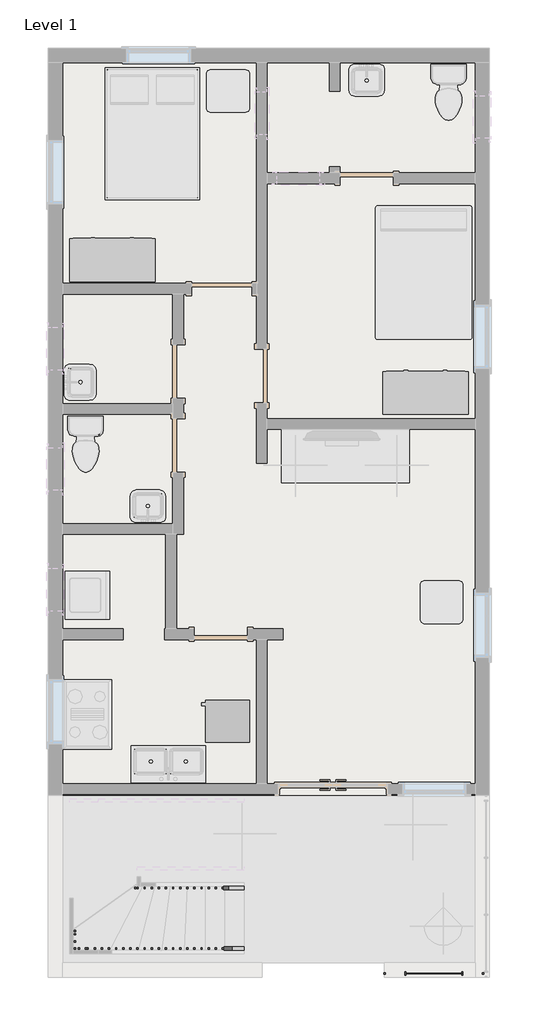
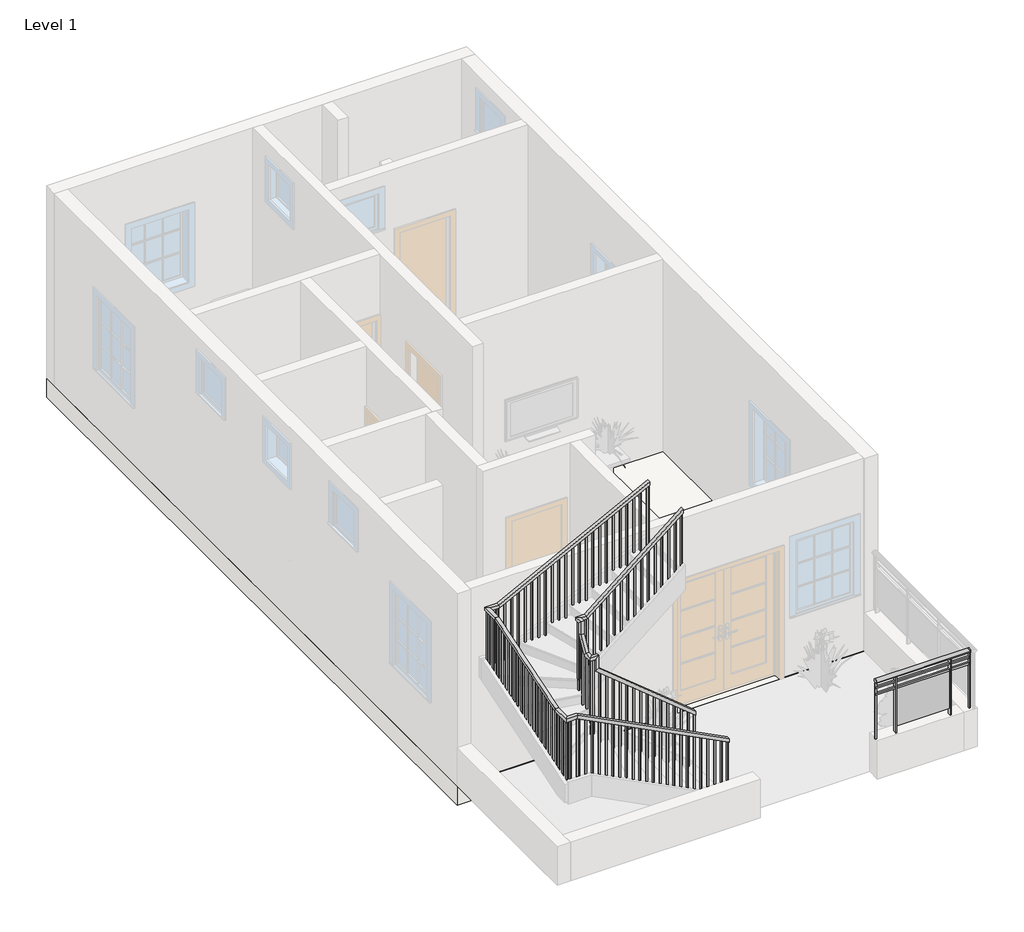
# One storey, part 2 of 3: 3 railings, 1 slab.
"""IFC4 building model written with IfcOpenShell, lengths in millimetres."""

from ifc_helpers import new_model, si_unit, point, frame, origin, place, context, project, spatial, polyline, ellipse_curve, trimmed, outline, extrude, faceted_brep, element, save
from ifc_brep_helpers import plane_surface, extruded_surface, advanced_brep

model = new_model("IFC4")

# Units and contexts
model_context = context("Model", 3, world=origin())
ifc_project = project(units=[si_unit("LENGTHUNIT", "METRE", prefix="MILLI")], contexts=[model_context])

# Site, building, storey
site = spatial("IfcSite", under=ifc_project)
building = spatial("IfcBuilding", under=site)
storey = spatial("IfcBuildingStorey", under=building, Name="Level 1", Elevation=0.0)

# Railings
placement = place(None, origin())
element("IfcRailing", 1, ObjectType="Glass Panel - Bottom Fill", at=placement, inside=storey, context=model_context, shape_type="SolidModel", body=[
    advanced_brep(
    [(-9850.6560632, 3087.8418963, 1524.0), (-9850.6560632, 3164.0418963, 1524.0), (-11259.7757671, 3087.8418963, 1524.0), (-11259.7757671, 3164.0418963, 1524.0)],
    [
        (0, 1, ellipse_curve(frame((-9850.6560632, 3125.9418963, 1524.0), z_axis=(1.0, 0.0, 0.0), x_axis=(0.0, 1.0, 0.0)), 38.1, 28.575)),
        (1, 0, ellipse_curve(frame((-9850.6560632, 3125.9418963, 1524.0), z_axis=(1.0, 0.0, 0.0), x_axis=(0.0, 1.0, 0.0)), 38.1, 28.575)),
        (2, 3, ellipse_curve(frame((-11259.7757671, 3125.9418963, 1524.0), z_axis=(-1.0, 0.0, 0.0), x_axis=(0.0, 1.0, 0.0)), 38.1, 28.575)),
        (3, 2, ellipse_curve(frame((-11259.7757671, 3125.9418963, 1524.0), z_axis=(-1.0, 0.0, 0.0), x_axis=(0.0, 1.0, 0.0)), 38.1, 28.575)),
        (0, 2),
        (3, 1),
    ],
    [
        plane_surface(frame((-9850.6560632, 3125.9418963, 1524.0), z_axis=(1.0, 0.0, 0.0), x_axis=(0.0, -1.0, 0.0))),
        plane_surface(frame((-11259.7757671, 3125.9418963, 1524.0), z_axis=(-1.0, 0.0, 0.0), x_axis=(0.0, -1.0, 0.0))),
        extruded_surface(trimmed(ellipse_curve(frame((-11259.7757671, 3125.9418963, 1524.0), z_axis=(1.0, 0.0, 0.0), x_axis=(0.0, 1.0, 0.0)), 38.1, 28.575), [point((-11259.7757671, 3087.8418963, 1524.0))], [point((-11259.7757671, 3164.0418963, 1524.0))], True, "CARTESIAN"), (1409.1197038999999, 0.0, 0.0), 1409.1197038999999),
        extruded_surface(trimmed(ellipse_curve(frame((-11259.7757671, 3125.9418963, 1524.0), z_axis=(1.0, 0.0, 0.0), x_axis=(0.0, 1.0, 0.0)), 38.1, 28.575), [point((-11259.7757671, 3164.0418963, 1524.0))], [point((-11259.7757671, 3087.8418963, 1524.0))], True, "CARTESIAN"), (1409.1197038999999, 0.0, 0.0), 1409.1197038999999),
    ],
    [
        (0, [[1, 2]]),
        (1, [[3, 4]]),
        (2, [[-1, 5, -4, 6]]),
        (3, [[-2, -6, -3, -5]]),
    ],
),
    extrude(outline(polyline([(-9850.6560632, 3138.6418963), (-9850.6560632, 3113.2418963), (-11259.7757671, 3113.2418963), (-11259.7757671, 3138.6418963), (-9850.6560632, 3138.6418963)])), frame((0.0, 0.0, 1409.7), z_axis=(0.0, 0.0, 1.0), x_axis=(1.0, 0.0, 0.0)), (0.0, 0.0, 1.0), 25.4),
    extrude(outline(polyline([(-9850.6560632, 3138.6418963), (-9850.6560632, 3113.2418963), (-11259.7757671, 3113.2418963), (-11259.7757671, 3138.6418963), (-9850.6560632, 3138.6418963)])), frame((0.0, 0.0, 1308.1), z_axis=(0.0, 0.0, 1.0), x_axis=(1.0, 0.0, 0.0)), (0.0, 0.0, 1.0), 25.4),
    extrude(outline(polyline([(-10955.2659151, 3151.3418963), (-10955.2659151, 3100.5418963), (-10967.9659151, 3100.5418963), (-10967.9659151, 3151.3418963), (-10955.2659151, 3151.3418963)])), frame((0.0, 0.0, 609.6), z_axis=(0.0, 0.0, 1.0), x_axis=(1.0, 0.0, 0.0)), (0.0, 0.0, 1.0), 885.6788223),
    extrude(outline(polyline([(-10148.8159151, 3119.4067393), (-10961.6159151, 3119.4067393), (-10961.6159151, 3125.7567393), (-10148.8159151, 3125.7567393), (-10148.8159151, 3119.4067393)])), frame((0.0, 0.0, 711.2), z_axis=(0.0, 0.0, 1.0), x_axis=(1.0, 0.0, 0.0)), (0.0, 0.0, 1.0), 596.9),
    extrude(outline(polyline([(-10142.4659151, 3151.3418963), (-10142.4659151, 3100.5418963), (-10155.1659151, 3100.5418963), (-10155.1659151, 3151.3418963), (-10142.4659151, 3151.3418963)])), frame((0.0, 0.0, 609.6), z_axis=(0.0, 0.0, 1.0), x_axis=(1.0, 0.0, 0.0)), (0.0, 0.0, 1.0), 885.6788223),
    extrude(outline(polyline([(-11247.0757671, 3135.4668963), (-11247.0757671, 3116.4168963), (-11266.1257671, 3116.4168963), (-11266.1257671, 3135.4668963), (-11247.0757671, 3135.4668963)])), frame((0.0, 0.0, 609.6), z_axis=(0.0, 0.0, 1.0), x_axis=(1.0, 0.0, 0.0)), (0.0, 0.0, 1.0), 885.6788223),
    extrude(outline(polyline([(-9844.3060632, 3135.4668963), (-9844.3060632, 3116.4168963), (-9863.3560632, 3116.4168963), (-9863.3560632, 3135.4668963), (-9844.3060632, 3135.4668963)])), frame((0.0, 0.0, 609.6), z_axis=(0.0, 0.0, 1.0), x_axis=(1.0, 0.0, 0.0)), (0.0, 0.0, 1.0), 885.6788223),
])
element("IfcRailing", 2, ObjectType="Handrail - Rectangular", at=placement, inside=storey, context=model_context, shape_type="SolidModel", body=[
    faceted_brep([(-13262.6440752, 4319.7418963, 1025.2529681), (-13262.6440752, 4319.7418963, 959.7067088), (-13262.6440752, 4370.5418963, 959.7067088), (-13262.6440752, 4370.5418963, 1025.2529681), (-14714.1757671, 4319.7418963, 2208.7848338), (-14764.9757671, 4319.7418963, 2184.659247), (-14764.9757671, 4370.5418963, 2184.659247), (-14714.1757671, 4370.5418963, 2208.7848338), (-14714.1757671, 4319.7418963, 2414.6281882), (-14764.9757671, 4319.7418963, 2363.8281882), (-14764.9757671, 4370.5418963, 2363.8281882), (-14714.1757671, 4370.5418963, 2414.6281882), (-14841.1757671, 4319.7418963, 2414.6281882), (-14841.1757671, 4319.7418963, 2363.8281882), (-14790.3757671, 4370.5418963, 2363.8281882), (-14790.3757671, 4370.5418963, 2414.6281882), (-14841.1757671, 4446.7418963, 2414.6281882), (-14841.1757671, 4475.8632301, 2363.8281882), (-14790.3757671, 4475.8632301, 2363.8281882), (-14790.3757671, 4446.7418963, 2414.6281882), (-14841.1757671, 4573.7418963, 2631.5051451), (-14841.1757671, 4624.5418963, 2617.7256424), (-14790.3757671, 4624.5418963, 2617.7256424), (-14790.3757671, 4573.7418963, 2631.5051451), (-14841.1757671, 4573.7418963, 2837.3484995), (-14841.1757671, 4624.5418963, 2786.5484995), (-14790.3757671, 4624.5418963, 2786.5484995), (-14790.3757671, 4573.7418963, 2837.3484995), (-14841.1757671, 4700.7418963, 2837.3484995), (-14841.1757671, 4700.7418963, 2786.5484995), (-14790.3757671, 4649.9418963, 2786.5484995), (-14790.3757671, 4649.9418963, 2837.3484995), (-14714.1757671, 4700.7418963, 2837.3484995), (-14696.090354, 4700.7418963, 2786.5484995), (-14696.090354, 4649.9418963, 2786.5484995), (-14714.1757671, 4649.9418963, 2837.3484995), (-13262.6440752, 4700.7418963, 4020.8803652), (-13262.6440752, 4649.9418963, 4020.8803652), (-13262.6440752, 4649.9418963, 3955.3341059), (-13262.6440752, 4700.7418963, 3955.3341059)], [[[0, 1, 2, 3]], [[1, 0, 4, 5]], [[2, 1, 5, 6]], [[3, 2, 6, 7]], [[0, 3, 7, 4]], [[5, 4, 8, 9]], [[6, 5, 9, 10]], [[7, 6, 10, 11]], [[4, 7, 11, 8]], [[9, 8, 12, 13]], [[10, 9, 13, 14]], [[11, 10, 14, 15]], [[8, 11, 15, 12]], [[13, 12, 16, 17]], [[14, 13, 17, 18]], [[15, 14, 18, 19]], [[12, 15, 19, 16]], [[17, 16, 20, 21]], [[18, 17, 21, 22]], [[19, 18, 22, 23]], [[16, 19, 23, 20]], [[21, 20, 24, 25]], [[22, 21, 25, 26]], [[23, 22, 26, 27]], [[20, 23, 27, 24]], [[25, 24, 28, 29]], [[26, 25, 29, 30]], [[27, 26, 30, 31]], [[24, 27, 31, 28]], [[29, 28, 32, 33]], [[30, 29, 33, 34]], [[31, 30, 34, 35]], [[28, 31, 35, 32]], [[36, 37, 38, 39]], [[33, 32, 36, 39]], [[34, 33, 39, 38]], [[35, 34, 38, 37]], [[32, 35, 37, 36]]]),
    extrude(outline(polyline([(3881.7558784, -13352.8834107), (3866.2231262, -13371.9334107), (2878.6666667, -13371.9334107), (2878.6666667, -13352.8834107), (3881.7558784, -13352.8834107)])), frame((0.0, 4665.8168963, 0.0), z_axis=(0.0, 1.0, 0.0), x_axis=(0.0, 0.0, 1.0)), (0.0, 0.0, 1.0), 19.05),
    extrude(outline(polyline([(3798.9145334, -13454.4834107), (3783.3817813, -13473.5334107), (2878.6666667, -13473.5334107), (2878.6666667, -13454.4834107), (3798.9145334, -13454.4834107)])), frame((0.0, 4665.8168963, 0.0), z_axis=(0.0, 1.0, 0.0), x_axis=(0.0, 0.0, 1.0)), (0.0, 0.0, 1.0), 19.05),
    extrude(outline(polyline([(3716.0731885, -13556.0834107), (3700.5404364, -13575.1334107), (2709.3333333, -13575.1334107), (2709.3333333, -13556.0834107), (3716.0731885, -13556.0834107)])), frame((0.0, 4665.8168963, 0.0), z_axis=(0.0, 1.0, 0.0), x_axis=(0.0, 0.0, 1.0)), (0.0, 0.0, 1.0), 19.05),
    extrude(outline(polyline([(3633.2318436, -13657.6834107), (3617.6990914, -13676.7334107), (2709.3333333, -13676.7334107), (2709.3333333, -13657.6834107), (3633.2318436, -13657.6834107)])), frame((0.0, 4665.8168963, 0.0), z_axis=(0.0, 1.0, 0.0), x_axis=(0.0, 0.0, 1.0)), (0.0, 0.0, 1.0), 19.05),
    extrude(outline(polyline([(3550.3904987, -13759.2834107), (3534.8577465, -13778.3334107), (2709.3333333, -13778.3334107), (2709.3333333, -13759.2834107), (3550.3904987, -13759.2834107)])), frame((0.0, 4665.8168963, 0.0), z_axis=(0.0, 1.0, 0.0), x_axis=(0.0, 0.0, 1.0)), (0.0, 0.0, 1.0), 19.05),
    extrude(outline(polyline([(3467.5491538, -13860.8834107), (3452.0164016, -13879.9334107), (2540.0, -13879.9334107), (2540.0, -13860.8834107), (3467.5491538, -13860.8834107)])), frame((0.0, 4665.8168963, 0.0), z_axis=(0.0, 1.0, 0.0), x_axis=(0.0, 0.0, 1.0)), (0.0, 0.0, 1.0), 19.05),
    extrude(outline(polyline([(3384.7078088, -13962.4834107), (3369.1750567, -13981.5334107), (2540.0, -13981.5334107), (2540.0, -13962.4834107), (3384.7078088, -13962.4834107)])), frame((0.0, 4665.8168963, 0.0), z_axis=(0.0, 1.0, 0.0), x_axis=(0.0, 0.0, 1.0)), (0.0, 0.0, 1.0), 19.05),
    extrude(outline(polyline([(3301.8664639, -14064.0834107), (3286.3337117, -14083.1334107), (2540.0, -14083.1334107), (2540.0, -14064.0834107), (3301.8664639, -14064.0834107)])), frame((0.0, 4665.8168963, 0.0), z_axis=(0.0, 1.0, 0.0), x_axis=(0.0, 0.0, 1.0)), (0.0, 0.0, 1.0), 19.05),
    extrude(outline(polyline([(3219.025119, -14165.6834107), (3203.4923668, -14184.7334107), (2370.6666667, -14184.7334107), (2370.6666667, -14165.6834107), (3219.025119, -14165.6834107)])), frame((0.0, 4665.8168963, 0.0), z_axis=(0.0, 1.0, 0.0), x_axis=(0.0, 0.0, 1.0)), (0.0, 0.0, 1.0), 19.05),
    extrude(outline(polyline([(3136.1837741, -14267.2834107), (3120.6510219, -14286.3334107), (2370.6666667, -14286.3334107), (2370.6666667, -14267.2834107), (3136.1837741, -14267.2834107)])), frame((0.0, 4665.8168963, 0.0), z_axis=(0.0, 1.0, 0.0), x_axis=(0.0, 0.0, 1.0)), (0.0, 0.0, 1.0), 19.05),
    extrude(outline(polyline([(3053.3424291, -14368.8834107), (3037.809677, -14387.9334107), (2201.3333333, -14387.9334107), (2201.3333333, -14368.8834107), (3053.3424291, -14368.8834107)])), frame((0.0, 4665.8168963, 0.0), z_axis=(0.0, 1.0, 0.0), x_axis=(0.0, 0.0, 1.0)), (0.0, 0.0, 1.0), 19.05),
    extrude(outline(polyline([(2970.5010842, -14470.4834107), (2954.9683321, -14489.5334107), (2201.3333333, -14489.5334107), (2201.3333333, -14470.4834107), (2970.5010842, -14470.4834107)])), frame((0.0, 4665.8168963, 0.0), z_axis=(0.0, 1.0, 0.0), x_axis=(0.0, 0.0, 1.0)), (0.0, 0.0, 1.0), 19.05),
    extrude(outline(polyline([(2887.6597393, -14572.0834107), (2872.1269871, -14591.1334107), (2032.0, -14591.1334107), (2032.0, -14572.0834107), (2887.6597393, -14572.0834107)])), frame((0.0, 4665.8168963, 0.0), z_axis=(0.0, 1.0, 0.0), x_axis=(0.0, 0.0, 1.0)), (0.0, 0.0, 1.0), 19.05),
    extrude(outline(polyline([(2804.8183944, -14673.6834107), (2789.2856422, -14692.7334107), (2032.0, -14692.7334107), (2032.0, -14673.6834107), (2804.8183944, -14673.6834107)])), frame((0.0, 4665.8168963, 0.0), z_axis=(0.0, 1.0, 0.0), x_axis=(0.0, 0.0, 1.0)), (0.0, 0.0, 1.0), 19.05),
    extrude(outline(polyline([(4553.6028, 2496.5834745), (4572.6528, 2529.115018), (4572.6528, 1524.0), (4553.6028, 1524.0), (4553.6028, 2496.5834745)])), frame((-14825.3007671, 0.0, 0.0), z_axis=(1.0, 0.0, 0.0), x_axis=(0.0, 1.0, 0.0)), (0.0, 0.0, 1.0), 19.05),
    extrude(outline(polyline([(4452.0028, 2323.0819089), (4471.0528, 2355.6134525), (4471.0528, 1524.0), (4452.0028, 1524.0), (4452.0028, 2323.0819089)])), frame((-14825.3007671, 0.0, 0.0), z_axis=(1.0, 0.0, 0.0), x_axis=(0.0, 1.0, 0.0)), (0.0, 0.0, 1.0), 19.05),
    extrude(outline(polyline([(2111.7191617, -14675.5190752), (2127.2519138, -14694.5690752), (1016.0, -14694.5690752), (1016.0, -14675.5190752), (2111.7191617, -14675.5190752)])), frame((0.0, 4335.6168963, 0.0), z_axis=(0.0, 1.0, 0.0), x_axis=(0.0, 0.0, 1.0)), (0.0, 0.0, 1.0), 19.05),
    extrude(outline(polyline([(2028.8778167, -14573.9190752), (2044.4105689, -14592.9690752), (1016.0, -14592.9690752), (1016.0, -14573.9190752), (2028.8778167, -14573.9190752)])), frame((0.0, 4335.6168963, 0.0), z_axis=(0.0, 1.0, 0.0), x_axis=(0.0, 0.0, 1.0)), (0.0, 0.0, 1.0), 19.05),
    extrude(outline(polyline([(1946.0364718, -14472.3190752), (1961.569224, -14491.3690752), (846.6666667, -14491.3690752), (846.6666667, -14472.3190752), (1946.0364718, -14472.3190752)])), frame((0.0, 4335.6168963, 0.0), z_axis=(0.0, 1.0, 0.0), x_axis=(0.0, 0.0, 1.0)), (0.0, 0.0, 1.0), 19.05),
    extrude(outline(polyline([(1863.1951269, -14370.7190752), (1878.7278791, -14389.7690752), (846.6666667, -14389.7690752), (846.6666667, -14370.7190752), (1863.1951269, -14370.7190752)])), frame((0.0, 4335.6168963, 0.0), z_axis=(0.0, 1.0, 0.0), x_axis=(0.0, 0.0, 1.0)), (0.0, 0.0, 1.0), 19.05),
    extrude(outline(polyline([(1780.353782, -14269.1190752), (1795.8865341, -14288.1690752), (677.3333333, -14288.1690752), (677.3333333, -14269.1190752), (1780.353782, -14269.1190752)])), frame((0.0, 4335.6168963, 0.0), z_axis=(0.0, 1.0, 0.0), x_axis=(0.0, 0.0, 1.0)), (0.0, 0.0, 1.0), 19.05),
    extrude(outline(polyline([(1697.5124371, -14167.5190752), (1713.0451892, -14186.5690752), (677.3333333, -14186.5690752), (677.3333333, -14167.5190752), (1697.5124371, -14167.5190752)])), frame((0.0, 4335.6168963, 0.0), z_axis=(0.0, 1.0, 0.0), x_axis=(0.0, 0.0, 1.0)), (0.0, 0.0, 1.0), 19.05),
    extrude(outline(polyline([(1614.6710921, -14065.9190752), (1630.2038443, -14084.9690752), (508.0, -14084.9690752), (508.0, -14065.9190752), (1614.6710921, -14065.9190752)])), frame((0.0, 4335.6168963, 0.0), z_axis=(0.0, 1.0, 0.0), x_axis=(0.0, 0.0, 1.0)), (0.0, 0.0, 1.0), 19.05),
    extrude(outline(polyline([(1531.8297472, -13964.3190752), (1547.3624994, -13983.3690752), (508.0, -13983.3690752), (508.0, -13964.3190752), (1531.8297472, -13964.3190752)])), frame((0.0, 4335.6168963, 0.0), z_axis=(0.0, 1.0, 0.0), x_axis=(0.0, 0.0, 1.0)), (0.0, 0.0, 1.0), 19.05),
    extrude(outline(polyline([(1448.9884023, -13862.7190752), (1464.5211545, -13881.7690752), (508.0, -13881.7690752), (508.0, -13862.7190752), (1448.9884023, -13862.7190752)])), frame((0.0, 4335.6168963, 0.0), z_axis=(0.0, 1.0, 0.0), x_axis=(0.0, 0.0, 1.0)), (0.0, 0.0, 1.0), 19.05),
    extrude(outline(polyline([(1366.1470574, -13761.1190752), (1381.6798095, -13780.1690752), (338.6666667, -13780.1690752), (338.6666667, -13761.1190752), (1366.1470574, -13761.1190752)])), frame((0.0, 4335.6168963, 0.0), z_axis=(0.0, 1.0, 0.0), x_axis=(0.0, 0.0, 1.0)), (0.0, 0.0, 1.0), 19.05),
    extrude(outline(polyline([(1283.3057124, -13659.5190752), (1298.8384646, -13678.5690752), (338.6666667, -13678.5690752), (338.6666667, -13659.5190752), (1283.3057124, -13659.5190752)])), frame((0.0, 4335.6168963, 0.0), z_axis=(0.0, 1.0, 0.0), x_axis=(0.0, 0.0, 1.0)), (0.0, 0.0, 1.0), 19.05),
    extrude(outline(polyline([(1200.4643675, -13557.9190752), (1215.9971197, -13576.9690752), (338.6666667, -13576.9690752), (338.6666667, -13557.9190752), (1200.4643675, -13557.9190752)])), frame((0.0, 4335.6168963, 0.0), z_axis=(0.0, 1.0, 0.0), x_axis=(0.0, 0.0, 1.0)), (0.0, 0.0, 1.0), 19.05),
    extrude(outline(polyline([(1117.6230226, -13456.3190752), (1133.1557748, -13475.3690752), (169.3333333, -13475.3690752), (169.3333333, -13456.3190752), (1117.6230226, -13456.3190752)])), frame((0.0, 4335.6168963, 0.0), z_axis=(0.0, 1.0, 0.0), x_axis=(0.0, 0.0, 1.0)), (0.0, 0.0, 1.0), 19.05),
    extrude(outline(polyline([(1034.7816777, -13354.7190752), (1050.3144298, -13373.7690752), (169.3333333, -13373.7690752), (169.3333333, -13354.7190752), (1034.7816777, -13354.7190752)])), frame((0.0, 4335.6168963, 0.0), z_axis=(0.0, 1.0, 0.0), x_axis=(0.0, 0.0, 1.0)), (0.0, 0.0, 1.0), 19.05),
    extrude(outline(polyline([(-14794.3334107, 4665.8168963), (-14794.3334107, 4684.8668963), (-14775.2834107, 4684.8668963), (-14775.2834107, 4665.8168963), (-14794.3334107, 4665.8168963)])), frame((0.0, 0.0, 1862.6666667), z_axis=(0.0, 0.0, 1.0), x_axis=(1.0, 0.0, 0.0)), (0.0, 0.0, 1.0), 923.8818329),
    extrude(outline(polyline([(-14806.2507671, 4665.8168963), (-14825.3007671, 4665.8168963), (-14825.3007671, 4684.8668963), (-14806.2507671, 4684.8668963), (-14806.2507671, 4665.8168963)])), frame((0.0, 0.0, 1862.6666667), z_axis=(0.0, 0.0, 1.0), x_axis=(1.0, 0.0, 0.0)), (0.0, 0.0, 1.0), 923.8818329),
    extrude(outline(polyline([(-14806.2507671, 4651.0309925), (-14825.3007671, 4651.0309925), (-14825.3007671, 4670.0809925), (-14806.2507671, 4670.0809925), (-14806.2507671, 4651.0309925)])), frame((0.0, 0.0, 1693.3333333), z_axis=(0.0, 0.0, 1.0), x_axis=(1.0, 0.0, 0.0)), (0.0, 0.0, 1.0), 1093.2151662),
    extrude(outline(polyline([(-14806.2507671, 4350.4028), (-14825.3007671, 4350.4028), (-14825.3007671, 4369.4528), (-14806.2507671, 4369.4528), (-14806.2507671, 4350.4028)])), frame((0.0, 0.0, 1354.6666667), z_axis=(0.0, 0.0, 1.0), x_axis=(1.0, 0.0, 0.0)), (0.0, 0.0, 1.0), 1009.1615215),
    extrude(outline(polyline([(-14806.2507671, 4354.6668963), (-14806.2507671, 4335.6168963), (-14825.3007671, 4335.6168963), (-14825.3007671, 4354.6668963), (-14806.2507671, 4354.6668963)])), frame((0.0, 0.0, 1185.3333333), z_axis=(0.0, 0.0, 1.0), x_axis=(1.0, 0.0, 0.0)), (0.0, 0.0, 1.0), 1178.4948549),
    extrude(outline(polyline([(-14775.2834107, 4354.6668963), (-14775.2834107, 4335.6168963), (-14794.3334107, 4335.6168963), (-14794.3334107, 4354.6668963), (-14775.2834107, 4354.6668963)])), frame((0.0, 0.0, 1185.3333333), z_axis=(0.0, 0.0, 1.0), x_axis=(1.0, 0.0, 0.0)), (0.0, 0.0, 1.0), 1178.4948549),
    extrude(outline(polyline([(3955.3341059, -13262.6440752), (3939.8013537, -13281.6940752), (2878.6666667, -13281.6940752), (2878.6666667, -13262.6440752), (3955.3341059, -13262.6440752)])), frame((0.0, 4665.8168963, 0.0), z_axis=(0.0, 1.0, 0.0), x_axis=(0.0, 0.0, 1.0)), (0.0, 0.0, 1.0), 19.05),
    extrude(outline(polyline([(959.7067088, -13262.6440752), (975.239461, -13281.6940752), (169.3333333, -13281.6940752), (169.3333333, -13262.6440752), (959.7067088, -13262.6440752)])), frame((0.0, 4335.6168963, 0.0), z_axis=(0.0, 1.0, 0.0), x_axis=(0.0, 0.0, 1.0)), (0.0, 0.0, 1.0), 19.05),
])
element("IfcRailing", 3, ObjectType="Handrail - Rectangular", at=placement, inside=storey, context=model_context, shape_type="SolidModel", body=[
    faceted_brep([(-13262.6440752, 3456.1418963, 1109.0771751), (-13262.6440752, 3456.1418963, 1051.9280057), (-13262.6440752, 3506.9418963, 1051.9280057), (-13262.6440752, 3506.9418963, 1109.0771751), (-15522.6259317, 3456.1418963, 2273.7644996), (-15534.945983, 3456.1418963, 2222.9644996), (-15534.945983, 3506.9418963, 2222.9644996), (-15522.6259317, 3506.9418963, 2273.7644996), (-15704.7757671, 3456.1418963, 2273.7644996), (-15704.7757671, 3456.1418963, 2222.9644996), (-15653.9757671, 3506.9418963, 2222.9644996), (-15653.9757671, 3506.9418963, 2273.7644996), (-15704.7757671, 3733.2958489, 2273.7644996), (-15704.7757671, 3741.246425, 2222.9644996), (-15653.9757671, 3741.246425, 2222.9644996), (-15653.9757671, 3733.2958489, 2273.7644996), (-15704.7757671, 5287.1879437, 2772.3688337), (-15704.7757671, 5295.1385198, 2721.5688337), (-15653.9757671, 5295.1385198, 2721.5688337), (-15653.9757671, 5287.1879437, 2772.3688337), (-15704.7757671, 5564.3418963, 2772.3688337), (-15704.7757671, 5564.3418963, 2721.5688337), (-15653.9757671, 5513.5418963, 2721.5688337), (-15653.9757671, 5513.5418963, 2772.3688337), (-15522.6259317, 5564.3418963, 2772.3688337), (-15510.3058804, 5564.3418963, 2721.5688337), (-15510.3058804, 5513.5418963, 2721.5688337), (-15522.6259317, 5513.5418963, 2772.3688337), (-13262.6440752, 5564.3418963, 3937.0561582), (-13262.6440752, 5513.5418963, 3937.0561582), (-13262.6440752, 5513.5418963, 3879.9069889), (-13262.6440752, 5564.3418963, 3879.9069889)], [[[0, 1, 2, 3]], [[1, 0, 4, 5]], [[2, 1, 5, 6]], [[3, 2, 6, 7]], [[0, 3, 7, 4]], [[5, 4, 8, 9]], [[6, 5, 9, 10]], [[7, 6, 10, 11]], [[4, 7, 11, 8]], [[9, 8, 12, 13]], [[10, 9, 13, 14]], [[11, 10, 14, 15]], [[8, 11, 15, 12]], [[13, 12, 16, 17]], [[14, 13, 17, 18]], [[15, 14, 18, 19]], [[12, 15, 19, 16]], [[17, 16, 20, 21]], [[18, 17, 21, 22]], [[19, 18, 22, 23]], [[16, 19, 23, 20]], [[21, 20, 24, 25]], [[22, 21, 25, 26]], [[23, 22, 26, 27]], [[20, 23, 27, 24]], [[28, 29, 30, 31]], [[25, 24, 28, 31]], [[26, 25, 31, 30]], [[27, 26, 30, 29]], [[24, 27, 29, 28]]]),
    extrude(outline(polyline([(3862.2268642, -13296.9509317), (2878.6666667, -13296.9509317), (2878.6666667, -13277.9009317), (3872.0443296, -13277.9009317), (3862.2268642, -13296.9509317)])), frame((0.0, 5529.4168963, 0.0), z_axis=(0.0, 1.0, 0.0), x_axis=(0.0, 0.0, 1.0)), (0.0, 0.0, 1.0), 19.05),
    extrude(outline(polyline([(3809.8670491, -13398.5509317), (2878.6666667, -13398.5509317), (2878.6666667, -13379.5009317), (3819.6845145, -13379.5009317), (3809.8670491, -13398.5509317)])), frame((0.0, 5529.4168963, 0.0), z_axis=(0.0, 1.0, 0.0), x_axis=(0.0, 0.0, 1.0)), (0.0, 0.0, 1.0), 19.05),
    extrude(outline(polyline([(3757.507234, -13500.1509317), (2878.6666667, -13500.1509317), (2878.6666667, -13481.1009317), (3767.3246993, -13481.1009317), (3757.507234, -13500.1509317)])), frame((0.0, 5529.4168963, 0.0), z_axis=(0.0, 1.0, 0.0), x_axis=(0.0, 0.0, 1.0)), (0.0, 0.0, 1.0), 19.05),
    extrude(outline(polyline([(3705.1474189, -13601.7509317), (2709.3333333, -13601.7509317), (2709.3333333, -13582.7009317), (3714.9648842, -13582.7009317), (3705.1474189, -13601.7509317)])), frame((0.0, 5529.4168963, 0.0), z_axis=(0.0, 1.0, 0.0), x_axis=(0.0, 0.0, 1.0)), (0.0, 0.0, 1.0), 19.05),
    extrude(outline(polyline([(3652.7876038, -13703.3509317), (2709.3333333, -13703.3509317), (2709.3333333, -13684.3009317), (3662.6050691, -13684.3009317), (3652.7876038, -13703.3509317)])), frame((0.0, 5529.4168963, 0.0), z_axis=(0.0, 1.0, 0.0), x_axis=(0.0, 0.0, 1.0)), (0.0, 0.0, 1.0), 19.05),
    extrude(outline(polyline([(3600.4277887, -13804.9509317), (2709.3333333, -13804.9509317), (2709.3333333, -13785.9009317), (3610.245254, -13785.9009317), (3600.4277887, -13804.9509317)])), frame((0.0, 5529.4168963, 0.0), z_axis=(0.0, 1.0, 0.0), x_axis=(0.0, 0.0, 1.0)), (0.0, 0.0, 1.0), 19.05),
    extrude(outline(polyline([(3548.0679735, -13906.5509317), (2540.0, -13906.5509317), (2540.0, -13887.5009317), (3557.8854389, -13887.5009317), (3548.0679735, -13906.5509317)])), frame((0.0, 5529.4168963, 0.0), z_axis=(0.0, 1.0, 0.0), x_axis=(0.0, 0.0, 1.0)), (0.0, 0.0, 1.0), 19.05),
    extrude(outline(polyline([(3495.7081584, -14008.1509317), (2540.0, -14008.1509317), (2540.0, -13989.1009317), (3505.5256238, -13989.1009317), (3495.7081584, -14008.1509317)])), frame((0.0, 5529.4168963, 0.0), z_axis=(0.0, 1.0, 0.0), x_axis=(0.0, 0.0, 1.0)), (0.0, 0.0, 1.0), 19.05),
    extrude(outline(polyline([(3443.3483433, -14109.7509317), (2540.0, -14109.7509317), (2540.0, -14090.7009317), (3453.1658086, -14090.7009317), (3443.3483433, -14109.7509317)])), frame((0.0, 5529.4168963, 0.0), z_axis=(0.0, 1.0, 0.0), x_axis=(0.0, 0.0, 1.0)), (0.0, 0.0, 1.0), 19.05),
    extrude(outline(polyline([(3390.9885282, -14211.3509317), (2370.6666667, -14211.3509317), (2370.6666667, -14192.3009317), (3400.8059935, -14192.3009317), (3390.9885282, -14211.3509317)])), frame((0.0, 5529.4168963, 0.0), z_axis=(0.0, 1.0, 0.0), x_axis=(0.0, 0.0, 1.0)), (0.0, 0.0, 1.0), 19.05),
    extrude(outline(polyline([(3338.6287131, -14312.9509317), (2370.6666667, -14312.9509317), (2370.6666667, -14293.9009317), (3348.4461784, -14293.9009317), (3338.6287131, -14312.9509317)])), frame((0.0, 5529.4168963, 0.0), z_axis=(0.0, 1.0, 0.0), x_axis=(0.0, 0.0, 1.0)), (0.0, 0.0, 1.0), 19.05),
    extrude(outline(polyline([(3286.268898, -14414.5509317), (2370.6666667, -14414.5509317), (2370.6666667, -14395.5009317), (3296.0863633, -14395.5009317), (3286.268898, -14414.5509317)])), frame((0.0, 5529.4168963, 0.0), z_axis=(0.0, 1.0, 0.0), x_axis=(0.0, 0.0, 1.0)), (0.0, 0.0, 1.0), 19.05),
    extrude(outline(polyline([(3233.9090828, -14516.1509317), (2201.3333333, -14516.1509317), (2201.3333333, -14497.1009317), (3243.7265482, -14497.1009317), (3233.9090828, -14516.1509317)])), frame((0.0, 5529.4168963, 0.0), z_axis=(0.0, 1.0, 0.0), x_axis=(0.0, 0.0, 1.0)), (0.0, 0.0, 1.0), 19.05),
    extrude(outline(polyline([(3181.5492677, -14617.7509317), (2201.3333333, -14617.7509317), (2201.3333333, -14598.7009317), (3191.3667331, -14598.7009317), (3181.5492677, -14617.7509317)])), frame((0.0, 5529.4168963, 0.0), z_axis=(0.0, 1.0, 0.0), x_axis=(0.0, 0.0, 1.0)), (0.0, 0.0, 1.0), 19.05),
    extrude(outline(polyline([(3129.1894526, -14719.3509317), (2201.3333333, -14719.3509317), (2201.3333333, -14700.3009317), (3139.0069179, -14700.3009317), (3129.1894526, -14719.3509317)])), frame((0.0, 5529.4168963, 0.0), z_axis=(0.0, 1.0, 0.0), x_axis=(0.0, 0.0, 1.0)), (0.0, 0.0, 1.0), 19.05),
    extrude(outline(polyline([(3076.8296375, -14820.9509317), (2032.0, -14820.9509317), (2032.0, -14801.9009317), (3086.6471028, -14801.9009317), (3076.8296375, -14820.9509317)])), frame((0.0, 5529.4168963, 0.0), z_axis=(0.0, 1.0, 0.0), x_axis=(0.0, 0.0, 1.0)), (0.0, 0.0, 1.0), 19.05),
    extrude(outline(polyline([(3024.4698224, -14922.5509317), (2032.0, -14922.5509317), (2032.0, -14903.5009317), (3034.2872877, -14903.5009317), (3024.4698224, -14922.5509317)])), frame((0.0, 5529.4168963, 0.0), z_axis=(0.0, 1.0, 0.0), x_axis=(0.0, 0.0, 1.0)), (0.0, 0.0, 1.0), 19.05),
    extrude(outline(polyline([(2972.1100073, -15024.1509317), (2032.0, -15024.1509317), (2032.0, -15005.1009317), (2981.9274726, -15005.1009317), (2972.1100073, -15024.1509317)])), frame((0.0, 5529.4168963, 0.0), z_axis=(0.0, 1.0, 0.0), x_axis=(0.0, 0.0, 1.0)), (0.0, 0.0, 1.0), 19.05),
    extrude(outline(polyline([(2919.7501921, -15125.7509317), (2032.0, -15125.7509317), (2032.0, -15106.7009317), (2929.5676575, -15106.7009317), (2919.7501921, -15125.7509317)])), frame((0.0, 5529.4168963, 0.0), z_axis=(0.0, 1.0, 0.0), x_axis=(0.0, 0.0, 1.0)), (0.0, 0.0, 1.0), 19.05),
    extrude(outline(polyline([(2867.390377, -15227.3509317), (1862.6666667, -15227.3509317), (1862.6666667, -15208.3009317), (2877.2078424, -15208.3009317), (2867.390377, -15227.3509317)])), frame((0.0, 5529.4168963, 0.0), z_axis=(0.0, 1.0, 0.0), x_axis=(0.0, 0.0, 1.0)), (0.0, 0.0, 1.0), 19.05),
    extrude(outline(polyline([(2815.0305619, -15328.9509317), (1862.6666667, -15328.9509317), (1862.6666667, -15309.9009317), (2824.8480272, -15309.9009317), (2815.0305619, -15328.9509317)])), frame((0.0, 5529.4168963, 0.0), z_axis=(0.0, 1.0, 0.0), x_axis=(0.0, 0.0, 1.0)), (0.0, 0.0, 1.0), 19.05),
    extrude(outline(polyline([(2762.6707468, -15430.5509317), (1862.6666667, -15430.5509317), (1862.6666667, -15411.5009317), (2772.4882121, -15411.5009317), (2762.6707468, -15430.5509317)])), frame((0.0, 5529.4168963, 0.0), z_axis=(0.0, 1.0, 0.0), x_axis=(0.0, 0.0, 1.0)), (0.0, 0.0, 1.0), 19.05),
    extrude(outline(polyline([(-15587.3007671, 5548.4668963), (-15568.2507671, 5548.4668963), (-15568.2507671, 5529.4168963), (-15587.3007671, 5529.4168963), (-15587.3007671, 5548.4668963)])), frame((0.0, 0.0, 1862.6666667), z_axis=(0.0, 0.0, 1.0), x_axis=(1.0, 0.0, 0.0)), (0.0, 0.0, 1.0), 858.902167),
    extrude(outline(polyline([(-15688.9007671, 5480.8629437), (-15688.9007671, 5499.9129437), (-15669.8507671, 5499.9129437), (-15669.8507671, 5480.8629437), (-15688.9007671, 5480.8629437)])), frame((0.0, 0.0, 1862.6666667), z_axis=(0.0, 0.0, 1.0), x_axis=(1.0, 0.0, 0.0)), (0.0, 0.0, 1.0), 858.902167),
    extrude(outline(polyline([(-15688.9007671, 5379.2629437), (-15688.9007671, 5398.3129437), (-15669.8507671, 5398.3129437), (-15669.8507671, 5379.2629437), (-15688.9007671, 5379.2629437)])), frame((0.0, 0.0, 1862.6666667), z_axis=(0.0, 0.0, 1.0), x_axis=(1.0, 0.0, 0.0)), (0.0, 0.0, 1.0), 858.902167),
    extrude(outline(polyline([(5266.8208489, 2712.4824155), (5266.8208489, 1693.3333333), (5247.7708489, 1693.3333333), (5247.7708489, 2706.3697564), (5266.8208489, 2712.4824155)])), frame((-15688.9007671, 0.0, 0.0), z_axis=(1.0, 0.0, 0.0), x_axis=(0.0, 1.0, 0.0)), (0.0, 0.0, 1.0), 19.05),
    extrude(outline(polyline([(5165.2208489, 2679.8815673), (5165.2208489, 1693.3333333), (5146.1708489, 1693.3333333), (5146.1708489, 2673.7689082), (5165.2208489, 2679.8815673)])), frame((-15688.9007671, 0.0, 0.0), z_axis=(1.0, 0.0, 0.0), x_axis=(0.0, 1.0, 0.0)), (0.0, 0.0, 1.0), 19.05),
    extrude(outline(polyline([(5063.6208489, 2647.280719), (5063.6208489, 1693.3333333), (5044.5708489, 1693.3333333), (5044.5708489, 2641.16806), (5063.6208489, 2647.280719)])), frame((-15688.9007671, 0.0, 0.0), z_axis=(1.0, 0.0, 0.0), x_axis=(0.0, 1.0, 0.0)), (0.0, 0.0, 1.0), 19.05),
    extrude(outline(polyline([(4962.0208489, 2614.6798708), (4962.0208489, 1693.3333333), (4942.9708489, 1693.3333333), (4942.9708489, 2608.5672118), (4962.0208489, 2614.6798708)])), frame((-15688.9007671, 0.0, 0.0), z_axis=(1.0, 0.0, 0.0), x_axis=(0.0, 1.0, 0.0)), (0.0, 0.0, 1.0), 19.05),
    extrude(outline(polyline([(4860.4208489, 2582.0790226), (4860.4208489, 1693.3333333), (4841.3708489, 1693.3333333), (4841.3708489, 2575.9663635), (4860.4208489, 2582.0790226)])), frame((-15688.9007671, 0.0, 0.0), z_axis=(1.0, 0.0, 0.0), x_axis=(0.0, 1.0, 0.0)), (0.0, 0.0, 1.0), 19.05),
    extrude(outline(polyline([(4758.8208489, 2549.4781744), (4758.8208489, 1693.3333333), (4739.7708489, 1693.3333333), (4739.7708489, 2543.3655153), (4758.8208489, 2549.4781744)])), frame((-15688.9007671, 0.0, 0.0), z_axis=(1.0, 0.0, 0.0), x_axis=(0.0, 1.0, 0.0)), (0.0, 0.0, 1.0), 19.05),
    extrude(outline(polyline([(4657.2208489, 2516.8773261), (4657.2208489, 1524.0), (4638.1708489, 1524.0), (4638.1708489, 2510.7646671), (4657.2208489, 2516.8773261)])), frame((-15688.9007671, 0.0, 0.0), z_axis=(1.0, 0.0, 0.0), x_axis=(0.0, 1.0, 0.0)), (0.0, 0.0, 1.0), 19.05),
    extrude(outline(polyline([(4555.6208489, 2484.2764779), (4555.6208489, 1524.0), (4536.5708489, 1524.0), (4536.5708489, 2478.1638189), (4555.6208489, 2484.2764779)])), frame((-15688.9007671, 0.0, 0.0), z_axis=(1.0, 0.0, 0.0), x_axis=(0.0, 1.0, 0.0)), (0.0, 0.0, 1.0), 19.05),
    extrude(outline(polyline([(4454.0208489, 2451.6756297), (4454.0208489, 1524.0), (4434.9708489, 1524.0), (4434.9708489, 2445.5629706), (4454.0208489, 2451.6756297)])), frame((-15688.9007671, 0.0, 0.0), z_axis=(1.0, 0.0, 0.0), x_axis=(0.0, 1.0, 0.0)), (0.0, 0.0, 1.0), 19.05),
    extrude(outline(polyline([(4352.4208489, 2419.0747814), (4352.4208489, 1524.0), (4333.3708489, 1524.0), (4333.3708489, 2412.9621224), (4352.4208489, 2419.0747814)])), frame((-15688.9007671, 0.0, 0.0), z_axis=(1.0, 0.0, 0.0), x_axis=(0.0, 1.0, 0.0)), (0.0, 0.0, 1.0), 19.05),
    extrude(outline(polyline([(4250.8208489, 2386.4739332), (4250.8208489, 1354.6666667), (4231.7708489, 1354.6666667), (4231.7708489, 2380.3612742), (4250.8208489, 2386.4739332)])), frame((-15688.9007671, 0.0, 0.0), z_axis=(1.0, 0.0, 0.0), x_axis=(0.0, 1.0, 0.0)), (0.0, 0.0, 1.0), 19.05),
    extrude(outline(polyline([(4149.2208489, 2353.873085), (4149.2208489, 1354.6666667), (4130.1708489, 1354.6666667), (4130.1708489, 2347.7604259), (4149.2208489, 2353.873085)])), frame((-15688.9007671, 0.0, 0.0), z_axis=(1.0, 0.0, 0.0), x_axis=(0.0, 1.0, 0.0)), (0.0, 0.0, 1.0), 19.05),
    extrude(outline(polyline([(4047.6208489, 2321.2722368), (4047.6208489, 1354.6666667), (4028.5708489, 1354.6666667), (4028.5708489, 2315.1595777), (4047.6208489, 2321.2722368)])), frame((-15688.9007671, 0.0, 0.0), z_axis=(1.0, 0.0, 0.0), x_axis=(0.0, 1.0, 0.0)), (0.0, 0.0, 1.0), 19.05),
    extrude(outline(polyline([(3946.0208489, 2288.6713885), (3946.0208489, 1354.6666667), (3926.9708489, 1354.6666667), (3926.9708489, 2282.5587295), (3946.0208489, 2288.6713885)])), frame((-15688.9007671, 0.0, 0.0), z_axis=(1.0, 0.0, 0.0), x_axis=(0.0, 1.0, 0.0)), (0.0, 0.0, 1.0), 19.05),
    extrude(outline(polyline([(3844.4208489, 2256.0705403), (3844.4208489, 1354.6666667), (3825.3708489, 1354.6666667), (3825.3708489, 2249.9578813), (3844.4208489, 2256.0705403)])), frame((-15688.9007671, 0.0, 0.0), z_axis=(1.0, 0.0, 0.0), x_axis=(0.0, 1.0, 0.0)), (0.0, 0.0, 1.0), 19.05),
    extrude(outline(polyline([(-15688.9007671, 3675.2168963), (-15688.9007671, 3694.2668963), (-15669.8507671, 3694.2668963), (-15669.8507671, 3675.2168963), (-15688.9007671, 3675.2168963)])), frame((0.0, 0.0, 1185.3333333), z_axis=(0.0, 0.0, 1.0), x_axis=(1.0, 0.0, 0.0)), (0.0, 0.0, 1.0), 1037.6311663),
    extrude(outline(polyline([(-15688.9007671, 3573.6168963), (-15688.9007671, 3592.6668963), (-15669.8507671, 3592.6668963), (-15669.8507671, 3573.6168963), (-15688.9007671, 3573.6168963)])), frame((0.0, 0.0, 1185.3333333), z_axis=(0.0, 0.0, 1.0), x_axis=(1.0, 0.0, 0.0)), (0.0, 0.0, 1.0), 1037.6311663),
    extrude(outline(polyline([(-15614.7009317, 3472.0168963), (-15633.7509317, 3472.0168963), (-15633.7509317, 3491.0668963), (-15614.7009317, 3491.0668963), (-15614.7009317, 3472.0168963)])), frame((0.0, 0.0, 1185.3333333), z_axis=(0.0, 0.0, 1.0), x_axis=(1.0, 0.0, 0.0)), (0.0, 0.0, 1.0), 1037.6311663),
    extrude(outline(polyline([(2208.752671, -15507.3690752), (1185.3333333, -15507.3690752), (1185.3333333, -15488.3190752), (2198.9352056, -15488.3190752), (2208.752671, -15507.3690752)])), frame((0.0, 3472.0168963, 0.0), z_axis=(0.0, 1.0, 0.0), x_axis=(0.0, 0.0, 1.0)), (0.0, 0.0, 1.0), 19.05),
    extrude(outline(polyline([(2156.3928558, -15405.7690752), (1185.3333333, -15405.7690752), (1185.3333333, -15386.7190752), (2146.5753905, -15386.7190752), (2156.3928558, -15405.7690752)])), frame((0.0, 3472.0168963, 0.0), z_axis=(0.0, 1.0, 0.0), x_axis=(0.0, 0.0, 1.0)), (0.0, 0.0, 1.0), 19.05),
    extrude(outline(polyline([(2104.0330407, -15304.1690752), (1185.3333333, -15304.1690752), (1185.3333333, -15285.1190752), (2094.2155754, -15285.1190752), (2104.0330407, -15304.1690752)])), frame((0.0, 3472.0168963, 0.0), z_axis=(0.0, 1.0, 0.0), x_axis=(0.0, 0.0, 1.0)), (0.0, 0.0, 1.0), 19.05),
    extrude(outline(polyline([(2051.6732256, -15202.5690752), (1185.3333333, -15202.5690752), (1185.3333333, -15183.5190752), (2041.8557603, -15183.5190752), (2051.6732256, -15202.5690752)])), frame((0.0, 3472.0168963, 0.0), z_axis=(0.0, 1.0, 0.0), x_axis=(0.0, 0.0, 1.0)), (0.0, 0.0, 1.0), 19.05),
    extrude(outline(polyline([(1999.3134105, -15100.9690752), (1016.0, -15100.9690752), (1016.0, -15081.9190752), (1989.4959452, -15081.9190752), (1999.3134105, -15100.9690752)])), frame((0.0, 3472.0168963, 0.0), z_axis=(0.0, 1.0, 0.0), x_axis=(0.0, 0.0, 1.0)), (0.0, 0.0, 1.0), 19.05),
    extrude(outline(polyline([(1946.9535954, -14999.3690752), (1016.0, -14999.3690752), (1016.0, -14980.3190752), (1937.13613, -14980.3190752), (1946.9535954, -14999.3690752)])), frame((0.0, 3472.0168963, 0.0), z_axis=(0.0, 1.0, 0.0), x_axis=(0.0, 0.0, 1.0)), (0.0, 0.0, 1.0), 19.05),
    extrude(outline(polyline([(1894.5937803, -14897.7690752), (1016.0, -14897.7690752), (1016.0, -14878.7190752), (1884.7763149, -14878.7190752), (1894.5937803, -14897.7690752)])), frame((0.0, 3472.0168963, 0.0), z_axis=(0.0, 1.0, 0.0), x_axis=(0.0, 0.0, 1.0)), (0.0, 0.0, 1.0), 19.05),
    extrude(outline(polyline([(1842.2339651, -14796.1690752), (1016.0, -14796.1690752), (1016.0, -14777.1190752), (1832.4164998, -14777.1190752), (1842.2339651, -14796.1690752)])), frame((0.0, 3472.0168963, 0.0), z_axis=(0.0, 1.0, 0.0), x_axis=(0.0, 0.0, 1.0)), (0.0, 0.0, 1.0), 19.05),
    extrude(outline(polyline([(1789.87415, -14694.5690752), (846.6666667, -14694.5690752), (846.6666667, -14675.5190752), (1780.0566847, -14675.5190752), (1789.87415, -14694.5690752)])), frame((0.0, 3472.0168963, 0.0), z_axis=(0.0, 1.0, 0.0), x_axis=(0.0, 0.0, 1.0)), (0.0, 0.0, 1.0), 19.05),
    extrude(outline(polyline([(1737.5143349, -14592.9690752), (846.6666667, -14592.9690752), (846.6666667, -14573.9190752), (1727.6968696, -14573.9190752), (1737.5143349, -14592.9690752)])), frame((0.0, 3472.0168963, 0.0), z_axis=(0.0, 1.0, 0.0), x_axis=(0.0, 0.0, 1.0)), (0.0, 0.0, 1.0), 19.05),
    extrude(outline(polyline([(1685.1545198, -14491.3690752), (846.6666667, -14491.3690752), (846.6666667, -14472.3190752), (1675.3370545, -14472.3190752), (1685.1545198, -14491.3690752)])), frame((0.0, 3472.0168963, 0.0), z_axis=(0.0, 1.0, 0.0), x_axis=(0.0, 0.0, 1.0)), (0.0, 0.0, 1.0), 19.05),
    extrude(outline(polyline([(1632.7947047, -14389.7690752), (677.3333333, -14389.7690752), (677.3333333, -14370.7190752), (1622.9772393, -14370.7190752), (1632.7947047, -14389.7690752)])), frame((0.0, 3472.0168963, 0.0), z_axis=(0.0, 1.0, 0.0), x_axis=(0.0, 0.0, 1.0)), (0.0, 0.0, 1.0), 19.05),
    extrude(outline(polyline([(1580.4348896, -14288.1690752), (677.3333333, -14288.1690752), (677.3333333, -14269.1190752), (1570.6174242, -14269.1190752), (1580.4348896, -14288.1690752)])), frame((0.0, 3472.0168963, 0.0), z_axis=(0.0, 1.0, 0.0), x_axis=(0.0, 0.0, 1.0)), (0.0, 0.0, 1.0), 19.05),
    extrude(outline(polyline([(1528.0750744, -14186.5690752), (677.3333333, -14186.5690752), (677.3333333, -14167.5190752), (1518.2576091, -14167.5190752), (1528.0750744, -14186.5690752)])), frame((0.0, 3472.0168963, 0.0), z_axis=(0.0, 1.0, 0.0), x_axis=(0.0, 0.0, 1.0)), (0.0, 0.0, 1.0), 19.05),
    extrude(outline(polyline([(1475.7152593, -14084.9690752), (508.0, -14084.9690752), (508.0, -14065.9190752), (1465.897794, -14065.9190752), (1475.7152593, -14084.9690752)])), frame((0.0, 3472.0168963, 0.0), z_axis=(0.0, 1.0, 0.0), x_axis=(0.0, 0.0, 1.0)), (0.0, 0.0, 1.0), 19.05),
    extrude(outline(polyline([(1423.3554442, -13983.3690752), (508.0, -13983.3690752), (508.0, -13964.3190752), (1413.5379789, -13964.3190752), (1423.3554442, -13983.3690752)])), frame((0.0, 3472.0168963, 0.0), z_axis=(0.0, 1.0, 0.0), x_axis=(0.0, 0.0, 1.0)), (0.0, 0.0, 1.0), 19.05),
    extrude(outline(polyline([(1370.9956291, -13881.7690752), (508.0, -13881.7690752), (508.0, -13862.7190752), (1361.1781638, -13862.7190752), (1370.9956291, -13881.7690752)])), frame((0.0, 3472.0168963, 0.0), z_axis=(0.0, 1.0, 0.0), x_axis=(0.0, 0.0, 1.0)), (0.0, 0.0, 1.0), 19.05),
    extrude(outline(polyline([(1318.635814, -13780.1690752), (338.6666667, -13780.1690752), (338.6666667, -13761.1190752), (1308.8183486, -13761.1190752), (1318.635814, -13780.1690752)])), frame((0.0, 3472.0168963, 0.0), z_axis=(0.0, 1.0, 0.0), x_axis=(0.0, 0.0, 1.0)), (0.0, 0.0, 1.0), 19.05),
    extrude(outline(polyline([(1266.2759989, -13678.5690752), (338.6666667, -13678.5690752), (338.6666667, -13659.5190752), (1256.4585335, -13659.5190752), (1266.2759989, -13678.5690752)])), frame((0.0, 3472.0168963, 0.0), z_axis=(0.0, 1.0, 0.0), x_axis=(0.0, 0.0, 1.0)), (0.0, 0.0, 1.0), 19.05),
    extrude(outline(polyline([(1213.9161837, -13576.9690752), (338.6666667, -13576.9690752), (338.6666667, -13557.9190752), (1204.0987184, -13557.9190752), (1213.9161837, -13576.9690752)])), frame((0.0, 3472.0168963, 0.0), z_axis=(0.0, 1.0, 0.0), x_axis=(0.0, 0.0, 1.0)), (0.0, 0.0, 1.0), 19.05),
    extrude(outline(polyline([(1161.5563686, -13475.3690752), (169.3333333, -13475.3690752), (169.3333333, -13456.3190752), (1151.7389033, -13456.3190752), (1161.5563686, -13475.3690752)])), frame((0.0, 3472.0168963, 0.0), z_axis=(0.0, 1.0, 0.0), x_axis=(0.0, 0.0, 1.0)), (0.0, 0.0, 1.0), 19.05),
    extrude(outline(polyline([(1109.1965535, -13373.7690752), (169.3333333, -13373.7690752), (169.3333333, -13354.7190752), (1099.3790882, -13354.7190752), (1109.1965535, -13373.7690752)])), frame((0.0, 3472.0168963, 0.0), z_axis=(0.0, 1.0, 0.0), x_axis=(0.0, 0.0, 1.0)), (0.0, 0.0, 1.0), 19.05),
    extrude(outline(polyline([(-15532.1509317, 5548.4668963), (-15513.1009317, 5548.4668963), (-15513.1009317, 5529.4168963), (-15532.1509317, 5529.4168963), (-15532.1509317, 5548.4668963)])), frame((0.0, 0.0, 1862.6666667), z_axis=(0.0, 0.0, 1.0), x_axis=(1.0, 0.0, 0.0)), (0.0, 0.0, 1.0), 858.902167),
    extrude(outline(polyline([(-15688.9007671, 5529.4168963), (-15688.9007671, 5548.4668963), (-15669.8507671, 5548.4668963), (-15669.8507671, 5529.4168963), (-15688.9007671, 5529.4168963)])), frame((0.0, 0.0, 1862.6666667), z_axis=(0.0, 0.0, 1.0), x_axis=(1.0, 0.0, 0.0)), (0.0, 0.0, 1.0), 858.902167),
    extrude(outline(polyline([(5296.7129437, 2722.0740262), (5296.7129437, 1862.6666667), (5277.6629437, 1862.6666667), (5277.6629437, 2715.9613671), (5296.7129437, 2722.0740262)])), frame((-15688.9007671, 0.0, 0.0), z_axis=(1.0, 0.0, 0.0), x_axis=(0.0, 1.0, 0.0)), (0.0, 0.0, 1.0), 19.05),
    extrude(outline(polyline([(-15688.9007671, 3723.7708489), (-15688.9007671, 3742.8208489), (-15669.8507671, 3742.8208489), (-15669.8507671, 3723.7708489), (-15688.9007671, 3723.7708489)])), frame((0.0, 0.0, 1185.3333333), z_axis=(0.0, 0.0, 1.0), x_axis=(1.0, 0.0, 0.0)), (0.0, 0.0, 1.0), 1037.6311663),
    extrude(outline(polyline([(-15669.8507671, 3472.0168963), (-15688.9007671, 3472.0168963), (-15688.9007671, 3491.0668963), (-15669.8507671, 3491.0668963), (-15669.8507671, 3472.0168963)])), frame((0.0, 0.0, 1185.3333333), z_axis=(0.0, 0.0, 1.0), x_axis=(1.0, 0.0, 0.0)), (0.0, 0.0, 1.0), 1037.6311663),
    extrude(outline(polyline([(2221.5240629, -15532.1509317), (1185.3333333, -15532.1509317), (1185.3333333, -15513.1009317), (2211.7065976, -15513.1009317), (2221.5240629, -15532.1509317)])), frame((0.0, 3472.0168963, 0.0), z_axis=(0.0, 1.0, 0.0), x_axis=(0.0, 0.0, 1.0)), (0.0, 0.0, 1.0), 19.05),
    extrude(outline(polyline([(3870.0895235, -13281.6940752), (2878.6666667, -13281.6940752), (2878.6666667, -13262.6440752), (3879.9069889, -13262.6440752), (3870.0895235, -13281.6940752)])), frame((0.0, 5529.4168963, 0.0), z_axis=(0.0, 1.0, 0.0), x_axis=(0.0, 0.0, 1.0)), (0.0, 0.0, 1.0), 19.05),
    extrude(outline(polyline([(1061.7454711, -13281.6940752), (169.3333333, -13281.6940752), (169.3333333, -13262.6440752), (1051.9280057, -13262.6440752), (1061.7454711, -13281.6940752)])), frame((0.0, 3472.0168963, 0.0), z_axis=(0.0, 1.0, 0.0), x_axis=(0.0, 0.0, 1.0)), (0.0, 0.0, 1.0), 19.05),
])

# Slab
element("IfcSlab", 4, ObjectType="Generic - 12\"", at=placement, inside=storey, context=model_context, shape_type="SweptSolid", body=[
    extrude(outline(polyline([(-9761.1757671, 16321.2418963), (-9761.1757671, 5665.9418963), (-16060.3757671, 5665.9418963), (-16060.3757671, 16321.2418963), (-9761.1757671, 16321.2418963)])), frame((0.0, 0.0, -304.8), z_axis=(0.0, 0.0, 1.0), x_axis=(1.0, 0.0, 0.0)), (0.0, 0.0, 1.0), 304.8),
])

save(model, "model.ifc")

# Revit data of these elements
# Type "Glass Panel - Bottom Fill"
#   Assembly Code = "C2010400"
#   built-in parameter 1008612 = 0.0416667 (stored number, unit not read)
#   built-in parameter 1008611 = 0.0416667 (stored number, unit not read)
#   built-in parameter 1008609 = 0.333333 (stored number, unit not read)
#   built-in parameter 1008604 = 0.166667 (stored number, unit not read)
#   built-in parameter 1008603 = 0.166667 (stored number, unit not read)
#   Railing Height = 3' - 0"
#   built-in parameter 1008630 = 2
#   built-in parameter 1008610 = 2
#   built-in parameter 1008618 = Baluster - Square : 3/4"
# Type "Handrail - Rectangular"
#   Assembly Code = "C2010400"
#   built-in parameter 1008612 = 0.0416667 (stored number, unit not read)
#   built-in parameter 1008611 = 0.0416667 (stored number, unit not read)
#   built-in parameter 1008609 = 0.333333 (stored number, unit not read)
#   built-in parameter 1008604 = 0.166667 (stored number, unit not read)
#   built-in parameter 1008603 = 0.166667 (stored number, unit not read)
#   Railing Height = 3' - 0"
#   built-in parameter 1008630 = 2
#   built-in parameter 1008610 = 2
#   built-in parameter 1008618 = Baluster - Square : 3/4"
# Type "Generic - 12\""
#   Assembly Code = "B1010"
#   Function = 0
#   Layers, outside or top first: 1' - 0" no material (function 1)
# Element 1 (IfcRailing, "Glass Panel - Bottom Fill")
#   built-in parameter 1008621 = 2 (stored number, unit not read)
#   Phase Created = New Construction
#   Materials on its faces: "Glass"
# Elements 2, 3 (IfcRailing, "Handrail - Rectangular")
#   Phase Created = New Construction
# Element 4 (IfcSlab, "Generic - 12\"")
#   Height Offset From Level = 0' - 0"
#   Phase Created = New Construction
#   Materials on its faces: "Default Floor"
# Materials
#   "Glass": class "Glass", colour RGB 0 128 192, transparency 0.75, Description = "Soda Lime Glass", Cost = 0
#   "Default Floor": colour RGB 128 128 128, transparency 0
